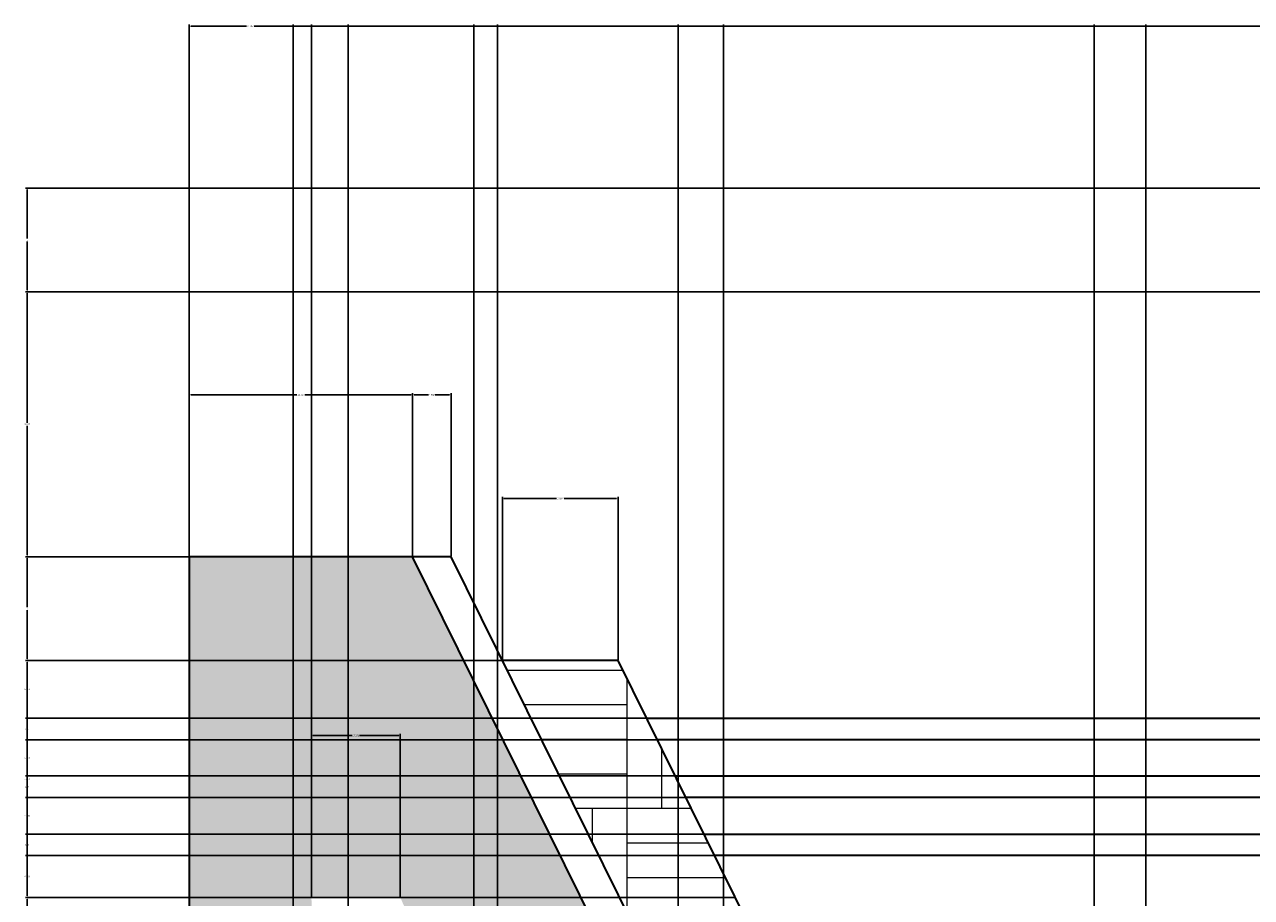
# Model space of a CAD drawing. Units: inches. Extents: x -9 to 389, y -55 to 344.
# Tile 3 of 5: x -9 to 133, y 243 to 344. Entities that reach past the tile are written whole.
import ezdxf

# ---------------------------------------------------------------- set-up
doc = ezdxf.new("R2010")
doc.units = ezdxf.units.IN
doc.header["$MEASUREMENT"] = 0
for name, color, linetype, lineweight in [('A-ANNO-DIMS', 2, 'Continuous', 18), ('A-ELEV', 7, 'Continuous', 35), ('A-ELEV-PATT', 8, 'Continuous', 13), ('A-ROOF', 1, 'Continuous', 35), ('A-ROOF-PATT', 8, 'Continuous', 13)]:
    doc.layers.add(name, color=color, linetype=linetype, lineweight=lineweight)
doc.styles.get("Standard").update_dxf_attribs({"font": 'arial.ttf'})
doc.dimstyles.get("Standard").update_dxf_attribs({"dimtxt": 0.18, "dimasz": 0.18, "dimexe": 0.18, "dimexo": 0.0625, "dimgap": 0.09, "dimtad": 0, "dimtih": 1, "dimtoh": 1, "dimdec": 4, "dimzin": 0, "dimdsep": 46, "dimtxsty": 'Standard', "dimcen": 0.09, "dimadec": 0, "dimazin": 0, "dimtfac": 1, "dimtdec": 4, "dimtofl": 0, "dimtmove": 0, "dimatfit": 3, "dimfxl": 1, "dimtolj": 1, "dimtzin": 0, "dimarcsym": 0})

# ---------------------------------------------------------------- blocks, each defined once
blk = doc.blocks.new('*D1')
at = {"layer": 'A-ANNO-DIMS', "color": 0, "lineweight": -2, "transparency": 16777216}
for p, q in [((9.65, 282.26), (9.65, 343.8)), ((9.83, 343.62), (16.26, 343.62)), ((23.59, 343.62), (17.17, 343.62)), ((23.77, 242.83), (23.77, 343.8))]:
    blk.add_line(p, q, dxfattribs=at)
at = {"layer": 'A-ANNO-DIMS', "color": 0, "transparency": 16777216}
for points in [[(9.83, 343.65), (9.83, 343.59), (9.65, 343.62)], [(23.59, 343.65), (23.59, 343.59), (23.77, 343.62)]]:
    blk.add_solid(points, dxfattribs=at)
at = {"layer": 'Defpoints', "color": 0, "transparency": 16777216}
for p in [(23.77, 343.62), (9.65, 282.2), (23.77, 242.77)]:
    blk.add_point(p, dxfattribs=at)
at = {"layer": 'A-ANNO-DIMS', "color": 0, "transparency": 16777216, "insert": (16.71, 343.62), "char_height": 0.18, "attachment_point": 5}
blk.add_mtext('\\A1;14.118', dxfattribs=at)
blk = doc.blocks.new('*D2')
at = {"layer": 'A-ANNO-DIMS', "color": 0, "lineweight": -2, "transparency": 16777216}
for p, q in [((23.77, 242.83), (23.77, 343.8)), ((23.95, 343.62), (25.5, 343.62)), ((27.83, 343.62), (26.29, 343.62)), ((28.01, 157.47), (28.01, 343.8))]:
    blk.add_line(p, q, dxfattribs=at)
at = {"layer": 'A-ANNO-DIMS', "color": 0, "transparency": 16777216}
for points in [[(23.95, 343.65), (23.95, 343.59), (23.77, 343.62)], [(27.83, 343.65), (27.83, 343.59), (28.01, 343.62)]]:
    blk.add_solid(points, dxfattribs=at)
at = {"layer": 'Defpoints', "color": 0, "transparency": 16777216}
for p in [(28.01, 343.62), (23.77, 242.77), (28.01, 157.4)]:
    blk.add_point(p, dxfattribs=at)
at = {"layer": 'A-ANNO-DIMS', "color": 0, "transparency": 16777216, "insert": (25.89, 343.62), "char_height": 0.18, "attachment_point": 5}
blk.add_mtext('\\A1;4.244', dxfattribs=at)
blk = doc.blocks.new('*D3')
at = {"layer": 'A-ANNO-DIMS', "color": 0, "lineweight": -2, "transparency": 16777216}
for p, q in [((28.01, 157.47), (28.01, 343.8)), ((28.19, 343.62), (49.26, 343.62)), ((71.27, 343.62), (50.2, 343.62)), ((71.45, 157.47), (71.45, 343.8))]:
    blk.add_line(p, q, dxfattribs=at)
at = {"layer": 'A-ANNO-DIMS', "color": 0, "transparency": 16777216}
for points in [[(28.19, 343.65), (28.19, 343.59), (28.01, 343.62)], [(71.27, 343.65), (71.27, 343.59), (71.45, 343.62)]]:
    blk.add_solid(points, dxfattribs=at)
at = {"layer": 'Defpoints', "color": 0, "transparency": 16777216}
for p in [(71.45, 343.62), (28.01, 157.4), (71.45, 157.4)]:
    blk.add_point(p, dxfattribs=at)
at = {"layer": 'A-ANNO-DIMS', "color": 0, "transparency": 16777216, "insert": (49.73, 343.62), "char_height": 0.18, "attachment_point": 5}
blk.add_mtext('\\A1;43.435', dxfattribs=at)
blk = doc.blocks.new('*D4')
at = {"layer": 'A-ANNO-DIMS', "color": 0, "lineweight": -2, "transparency": 16777216}
for p, q in [((71.45, 157.47), (71.45, 343.8)), ((71.63, 343.62), (119.03, 343.62)), ((167.08, 343.62), (119.68, 343.62)), ((167.26, 324.93), (167.26, 343.8))]:
    blk.add_line(p, q, dxfattribs=at)
at = {"layer": 'A-ANNO-DIMS', "color": 0, "transparency": 16777216}
for points in [[(71.63, 343.65), (71.63, 343.59), (71.45, 343.62)], [(167.08, 343.65), (167.08, 343.59), (167.26, 343.62)]]:
    blk.add_solid(points, dxfattribs=at)
at = {"layer": 'Defpoints', "color": 0, "transparency": 16777216}
for p in [(167.26, 343.62), (167.26, 324.87), (71.45, 157.4)]:
    blk.add_point(p, dxfattribs=at)
at = {"layer": 'A-ANNO-DIMS', "color": 0, "transparency": 16777216, "insert": (119.35, 343.62), "char_height": 0.18, "attachment_point": 5}
blk.add_mtext('\\A1;95.8', dxfattribs=at)
blk = doc.blocks.new('*D16')
at = {"layer": 'A-ANNO-DIMS', "color": 0, "lineweight": -2, "transparency": 16777216}
for p, q in [((21.65, 14.83), (21.65, 343.8)), ((21.83, 343.62), (31.64, 343.62)), ((42.37, 343.62), (32.57, 343.62)), ((42.55, 14.83), (42.55, 343.8))]:
    blk.add_line(p, q, dxfattribs=at)
at = {"layer": 'A-ANNO-DIMS', "color": 0, "transparency": 16777216}
for points in [[(21.83, 343.65), (21.83, 343.59), (21.65, 343.62)], [(42.37, 343.65), (42.37, 343.59), (42.55, 343.62)]]:
    blk.add_solid(points, dxfattribs=at)
at = {"layer": 'Defpoints', "color": 0, "transparency": 16777216}
for p in [(42.55, 343.62), (21.65, 14.77), (42.55, 14.77)]:
    blk.add_point(p, dxfattribs=at)
at = {"layer": 'A-ANNO-DIMS', "color": 0, "transparency": 16777216, "insert": (32.1, 343.62), "char_height": 0.18, "attachment_point": 5}
blk.add_mtext('\\A1;20.896', dxfattribs=at)
blk = doc.blocks.new('*D17')
at = {"layer": 'A-ANNO-DIMS', "color": 0, "lineweight": -2, "transparency": 16777216}
for p, q in [((42.55, 14.83), (42.55, 343.8)), ((42.73, 343.62), (43.61, 343.62)), ((45.14, 343.62), (44.26, 343.62)), ((45.32, 14.83), (45.32, 343.8))]:
    blk.add_line(p, q, dxfattribs=at)
at = {"layer": 'A-ANNO-DIMS', "color": 0, "transparency": 16777216}
for points in [[(42.73, 343.65), (42.73, 343.59), (42.55, 343.62)], [(45.14, 343.65), (45.14, 343.59), (45.32, 343.62)]]:
    blk.add_solid(points, dxfattribs=at)
at = {"layer": 'Defpoints', "color": 0, "transparency": 16777216}
for p in [(45.32, 343.62), (42.55, 14.77), (45.32, 14.77)]:
    blk.add_point(p, dxfattribs=at)
at = {"layer": 'A-ANNO-DIMS', "color": 0, "transparency": 16777216, "insert": (43.93, 343.62), "char_height": 0.18, "attachment_point": 5}
blk.add_mtext('\\A1;2.77', dxfattribs=at)
blk = doc.blocks.new('*D18')
at = {"layer": 'A-ANNO-DIMS', "color": 0, "lineweight": -2, "transparency": 16777216}
for p, q in [((45.32, 14.83), (45.32, 343.8)), ((45.5, 343.62), (55.3, 343.62)), ((66.03, 343.62), (56.23, 343.62)), ((66.21, 14.83), (66.21, 343.8))]:
    blk.add_line(p, q, dxfattribs=at)
at = {"layer": 'A-ANNO-DIMS', "color": 0, "transparency": 16777216}
for points in [[(45.5, 343.65), (45.5, 343.59), (45.32, 343.62)], [(66.03, 343.65), (66.03, 343.59), (66.21, 343.62)]]:
    blk.add_solid(points, dxfattribs=at)
at = {"layer": 'Defpoints', "color": 0, "transparency": 16777216}
for p in [(66.21, 343.62), (45.32, 14.77), (66.21, 14.77)]:
    blk.add_point(p, dxfattribs=at)
at = {"layer": 'A-ANNO-DIMS', "color": 0, "transparency": 16777216, "insert": (55.77, 343.62), "char_height": 0.18, "attachment_point": 5}
blk.add_mtext('\\A1;20.896', dxfattribs=at)
blk = doc.blocks.new('*D19')
at = {"layer": 'A-ANNO-DIMS', "color": 0, "lineweight": -2, "transparency": 16777216}
for p, q in [((66.21, 14.83), (66.21, 343.8)), ((66.39, 343.62), (109.71, 343.62)), ((153.81, 343.62), (110.5, 343.62)), ((153.99, 14.83), (153.99, 343.8))]:
    blk.add_line(p, q, dxfattribs=at)
at = {"layer": 'A-ANNO-DIMS', "color": 0, "transparency": 16777216}
for points in [[(66.39, 343.65), (66.39, 343.59), (66.21, 343.62)], [(153.81, 343.65), (153.81, 343.59), (153.99, 343.62)]]:
    blk.add_solid(points, dxfattribs=at)
at = {"layer": 'Defpoints', "color": 0, "transparency": 16777216}
for p in [(153.99, 343.62), (66.21, 14.77), (153.99, 14.77)]:
    blk.add_point(p, dxfattribs=at)
at = {"layer": 'A-ANNO-DIMS', "color": 0, "transparency": 16777216, "insert": (110.1, 343.62), "char_height": 0.18, "attachment_point": 5}
blk.add_mtext('\\A1;87.77', dxfattribs=at)
blk = doc.blocks.new('*D25')
at = {"layer": 'A-ANNO-DIMS', "color": 0, "lineweight": -2, "transparency": 16777216}
for p, q in [((23.71, 242.77), (-9.28, 242.77)), ((-9.1, 242.59), (-9.1, 200.27)), ((-9.1, 157.58), (-9.1, 199.9)), ((27.95, 157.4), (-9.28, 157.4))]:
    blk.add_line(p, q, dxfattribs=at)
at = {"layer": 'A-ANNO-DIMS', "color": 0, "transparency": 16777216}
for points in [[(-9.13, 242.59), (-9.07, 242.59), (-9.1, 242.77)], [(-9.13, 157.58), (-9.07, 157.58), (-9.1, 157.4)]]:
    blk.add_solid(points, dxfattribs=at)
at = {"layer": 'Defpoints', "color": 0, "transparency": 16777216}
for p in [(-9.1, 242.77), (23.77, 242.77), (28.01, 157.4)]:
    blk.add_point(p, dxfattribs=at)
at = {"layer": 'A-ANNO-DIMS', "color": 0, "transparency": 16777216, "insert": (-9.1, 200.09), "char_height": 0.18, "attachment_point": 5}
blk.add_mtext('\\A1;85.36', dxfattribs=at)
blk = doc.blocks.new('*D26')
at = {"layer": 'A-ANNO-DIMS', "color": 0, "lineweight": -2, "transparency": 16777216}
for p, q in [((59.2, 270.2), (-9.28, 270.2)), ((-9.1, 270.02), (-9.1, 256.67)), ((-9.1, 242.95), (-9.1, 256.3)), ((23.71, 242.77), (-9.28, 242.77))]:
    blk.add_line(p, q, dxfattribs=at)
at = {"layer": 'A-ANNO-DIMS', "color": 0, "transparency": 16777216}
for points in [[(-9.13, 270.02), (-9.07, 270.02), (-9.1, 270.2)], [(-9.13, 242.95), (-9.07, 242.95), (-9.1, 242.77)]]:
    blk.add_solid(points, dxfattribs=at)
at = {"layer": 'Defpoints', "color": 0, "transparency": 16777216}
for p in [(-9.1, 270.2), (59.26, 270.2), (23.77, 242.77)]:
    blk.add_point(p, dxfattribs=at)
at = {"layer": 'A-ANNO-DIMS', "color": 0, "transparency": 16777216, "insert": (-9.1, 256.48), "char_height": 0.18, "attachment_point": 5}
blk.add_mtext('\\A1;27.43', dxfattribs=at)
blk = doc.blocks.new('*D27')
at = {"layer": 'A-ANNO-DIMS', "color": 0, "lineweight": -2, "transparency": 16777216}
for p, q in [((9.59, 282.2), (-9.28, 282.2)), ((-9.1, 282.02), (-9.1, 276.38)), ((-9.1, 270.38), (-9.1, 276.02)), ((59.2, 270.2), (-9.28, 270.2))]:
    blk.add_line(p, q, dxfattribs=at)
at = {"layer": 'A-ANNO-DIMS', "color": 0, "transparency": 16777216}
for points in [[(-9.13, 282.02), (-9.07, 282.02), (-9.1, 282.2)], [(-9.13, 270.38), (-9.07, 270.38), (-9.1, 270.2)]]:
    blk.add_solid(points, dxfattribs=at)
at = {"layer": 'Defpoints', "color": 0, "transparency": 16777216}
for p in [(-9.1, 282.2), (9.65, 282.2), (59.26, 270.2)]:
    blk.add_point(p, dxfattribs=at)
at = {"layer": 'A-ANNO-DIMS', "color": 0, "transparency": 16777216, "insert": (-9.1, 276.2), "char_height": 0.18, "attachment_point": 5}
blk.add_mtext('\\A1;12', dxfattribs=at)
blk = doc.blocks.new('*D28')
at = {"layer": 'A-ANNO-DIMS', "color": 0, "lineweight": -2, "transparency": 16777216}
for p, q in [((160.42, 312.87), (-9.28, 312.87)), ((-9.1, 312.69), (-9.1, 297.72)), ((-9.1, 282.38), (-9.1, 297.35)), ((9.59, 282.2), (-9.28, 282.2))]:
    blk.add_line(p, q, dxfattribs=at)
at = {"layer": 'A-ANNO-DIMS', "color": 0, "transparency": 16777216}
for points in [[(-9.13, 312.69), (-9.07, 312.69), (-9.1, 312.87)], [(-9.13, 282.38), (-9.07, 282.38), (-9.1, 282.2)]]:
    blk.add_solid(points, dxfattribs=at)
at = {"layer": 'Defpoints', "color": 0, "transparency": 16777216}
for p in [(-9.1, 312.87), (160.49, 312.87), (9.65, 282.2)]:
    blk.add_point(p, dxfattribs=at)
at = {"layer": 'A-ANNO-DIMS', "color": 0, "transparency": 16777216, "insert": (-9.1, 297.54), "char_height": 0.18, "attachment_point": 5}
blk.add_mtext('\\A1;30.67', dxfattribs=at)
blk = doc.blocks.new('*D29')
at = {"layer": 'A-ANNO-DIMS', "color": 0, "lineweight": -2, "transparency": 16777216}
for p, q in [((369.59, 324.87), (-9.28, 324.87)), ((-9.1, 324.69), (-9.1, 319.05)), ((-9.1, 313.05), (-9.1, 318.69)), ((160.42, 312.87), (-9.28, 312.87))]:
    blk.add_line(p, q, dxfattribs=at)
at = {"layer": 'A-ANNO-DIMS', "color": 0, "transparency": 16777216}
for points in [[(-9.13, 324.69), (-9.07, 324.69), (-9.1, 324.87)], [(-9.13, 313.05), (-9.07, 313.05), (-9.1, 312.87)]]:
    blk.add_solid(points, dxfattribs=at)
at = {"layer": 'Defpoints', "color": 0, "transparency": 16777216}
for p in [(-9.1, 324.87), (369.65, 324.87), (160.49, 312.87)]:
    blk.add_point(p, dxfattribs=at)
at = {"layer": 'A-ANNO-DIMS', "color": 0, "transparency": 16777216, "insert": (-9.1, 318.87), "char_height": 0.18, "attachment_point": 5}
blk.add_mtext('\\A1;12', dxfattribs=at)
blk = doc.blocks.new('*D34')
at = {"layer": 'A-ANNO-DIMS', "color": 0, "lineweight": -2, "transparency": 16777216}
for p, q in [((9.65, 282.26), (9.65, 301.13)), ((9.83, 300.95), (22.1, 300.95)), ((35.3, 300.95), (23.03, 300.95)), ((35.48, 282.26), (35.48, 301.13))]:
    blk.add_line(p, q, dxfattribs=at)
at = {"layer": 'A-ANNO-DIMS', "color": 0, "transparency": 16777216}
for points in [[(9.83, 300.98), (9.83, 300.92), (9.65, 300.95)], [(35.3, 300.98), (35.3, 300.92), (35.48, 300.95)]]:
    blk.add_solid(points, dxfattribs=at)
at = {"layer": 'Defpoints', "color": 0, "transparency": 16777216}
for p in [(35.48, 300.95), (9.65, 282.2), (35.48, 282.2)]:
    blk.add_point(p, dxfattribs=at)
at = {"layer": 'A-ANNO-DIMS', "color": 0, "transparency": 16777216, "insert": (22.57, 300.95), "char_height": 0.18, "attachment_point": 5}
blk.add_mtext('\\A1;25.825', dxfattribs=at)
blk = doc.blocks.new('*D35')
at = {"layer": 'A-ANNO-DIMS', "color": 0, "lineweight": -2, "transparency": 16777216}
for p, q in [((35.48, 282.26), (35.48, 301.13)), ((35.66, 300.95), (37.31, 300.95)), ((39.76, 300.95), (38.11, 300.95)), ((39.94, 282.26), (39.94, 301.13))]:
    blk.add_line(p, q, dxfattribs=at)
at = {"layer": 'A-ANNO-DIMS', "color": 0, "transparency": 16777216}
for points in [[(35.66, 300.98), (35.66, 300.92), (35.48, 300.95)], [(39.76, 300.98), (39.76, 300.92), (39.94, 300.95)]]:
    blk.add_solid(points, dxfattribs=at)
at = {"layer": 'Defpoints', "color": 0, "transparency": 16777216}
for p in [(39.94, 300.95), (35.48, 282.2), (39.94, 282.2)]:
    blk.add_point(p, dxfattribs=at)
at = {"layer": 'A-ANNO-DIMS', "color": 0, "transparency": 16777216, "insert": (37.71, 300.95), "char_height": 0.18, "attachment_point": 5}
blk.add_mtext('\\A1;4.462', dxfattribs=at)
blk = doc.blocks.new('*D37')
at = {"layer": 'A-ANNO-DIMS', "color": 0, "lineweight": -2, "transparency": 16777216}
for p, q in [((45.87, 270.26), (45.87, 289.13)), ((46.05, 288.95), (52.11, 288.95)), ((59.08, 288.95), (53.02, 288.95)), ((59.26, 270.26), (59.26, 289.13))]:
    blk.add_line(p, q, dxfattribs=at)
at = {"layer": 'A-ANNO-DIMS', "color": 0, "transparency": 16777216}
for points in [[(46.05, 288.98), (46.05, 288.92), (45.87, 288.95)], [(59.08, 288.98), (59.08, 288.92), (59.26, 288.95)]]:
    blk.add_solid(points, dxfattribs=at)
at = {"layer": 'Defpoints', "color": 0, "transparency": 16777216}
for p in [(59.26, 288.95), (45.87, 270.2), (59.26, 270.2)]:
    blk.add_point(p, dxfattribs=at)
at = {"layer": 'A-ANNO-DIMS', "color": 0, "transparency": 16777216, "insert": (52.57, 288.95), "char_height": 0.18, "attachment_point": 5}
blk.add_mtext('\\A1;13.387', dxfattribs=at)
blk = doc.blocks.new('*D39')
at = {"layer": 'A-ANNO-DIMS', "color": 0, "lineweight": -2, "transparency": 16777216}
for p, q in [((23.77, 242.83), (23.77, 261.7)), ((23.95, 261.52), (28.48, 261.52)), ((33.88, 261.52), (29.35, 261.52)), ((34.06, 242.83), (34.06, 261.7))]:
    blk.add_line(p, q, dxfattribs=at)
at = {"layer": 'A-ANNO-DIMS', "color": 0, "transparency": 16777216}
for points in [[(23.95, 261.55), (23.95, 261.49), (23.77, 261.52)], [(33.88, 261.55), (33.88, 261.49), (34.06, 261.52)]]:
    blk.add_solid(points, dxfattribs=at)
at = {"layer": 'Defpoints', "color": 0, "transparency": 16777216}
for p in [(34.06, 261.52), (23.77, 242.77), (34.06, 242.77)]:
    blk.add_point(p, dxfattribs=at)
at = {"layer": 'A-ANNO-DIMS', "color": 0, "transparency": 16777216, "insert": (28.92, 261.52), "char_height": 0.18, "attachment_point": 5}
blk.add_mtext('\\A1;10.291', dxfattribs=at)
blk = doc.blocks.new('*D49')
at = {"layer": 'A-ANNO-DIMS', "color": 0, "lineweight": -2, "transparency": 16777216}
for p, q in [((72.76, 242.77), (-9.28, 242.77)), ((-9.1, 242.59), (-9.1, 232.95)), ((-9.1, 222.95), (-9.1, 232.59)), ((82.66, 222.77), (-9.28, 222.77))]:
    blk.add_line(p, q, dxfattribs=at)
at = {"layer": 'A-ANNO-DIMS', "color": 0, "transparency": 16777216}
for points in [[(-9.13, 242.59), (-9.07, 242.59), (-9.1, 242.77)], [(-9.13, 222.95), (-9.07, 222.95), (-9.1, 222.77)]]:
    blk.add_solid(points, dxfattribs=at)
at = {"layer": 'Defpoints', "color": 0, "transparency": 16777216}
for p in [(-9.1, 242.77), (72.83, 242.77), (82.72, 222.77)]:
    blk.add_point(p, dxfattribs=at)
at = {"layer": 'A-ANNO-DIMS', "color": 0, "transparency": 16777216, "insert": (-9.1, 232.77), "char_height": 0.18, "attachment_point": 5}
blk.add_mtext('\\A1;20', dxfattribs=at)
blk = doc.blocks.new('*D50')
at = {"layer": 'A-ANNO-DIMS', "color": 0, "lineweight": -2, "transparency": 16777216}
for p, q in [((70.37, 247.61), (-9.28, 247.61)), ((-9.1, 247.43), (-9.1, 245.37)), ((-9.1, 242.95), (-9.1, 245.01)), ((72.76, 242.77), (-9.28, 242.77))]:
    blk.add_line(p, q, dxfattribs=at)
at = {"layer": 'A-ANNO-DIMS', "color": 0, "transparency": 16777216}
for points in [[(-9.13, 247.43), (-9.07, 247.43), (-9.1, 247.61)], [(-9.13, 242.95), (-9.07, 242.95), (-9.1, 242.77)]]:
    blk.add_solid(points, dxfattribs=at)
at = {"layer": 'Defpoints', "color": 0, "transparency": 16777216}
for p in [(-9.1, 247.61), (70.43, 247.61), (72.83, 242.77)]:
    blk.add_point(p, dxfattribs=at)
at = {"layer": 'A-ANNO-DIMS', "color": 0, "transparency": 16777216, "insert": (-9.1, 245.19), "char_height": 0.18, "attachment_point": 5}
blk.add_mtext('\\A1;4.843', dxfattribs=at)
blk = doc.blocks.new('*D51')
at = {"layer": 'A-ANNO-DIMS', "color": 0, "lineweight": -2, "transparency": 16777216}
for p, q in [((69.13, 250.11), (-9.28, 250.11)), ((-9.1, 249.93), (-9.1, 249.04)), ((-9.1, 247.79), (-9.1, 248.68)), ((70.37, 247.61), (-9.28, 247.61))]:
    blk.add_line(p, q, dxfattribs=at)
at = {"layer": 'A-ANNO-DIMS', "color": 0, "transparency": 16777216}
for points in [[(-9.13, 249.93), (-9.07, 249.93), (-9.1, 250.11)], [(-9.13, 247.79), (-9.07, 247.79), (-9.1, 247.61)]]:
    blk.add_solid(points, dxfattribs=at)
at = {"layer": 'Defpoints', "color": 0, "transparency": 16777216}
for p in [(-9.1, 250.11), (69.19, 250.11), (70.43, 247.61)]:
    blk.add_point(p, dxfattribs=at)
at = {"layer": 'A-ANNO-DIMS', "color": 0, "transparency": 16777216, "insert": (-9.1, 248.86), "char_height": 0.18, "attachment_point": 5}
blk.add_mtext('\\A1;2.50', dxfattribs=at)
blk = doc.blocks.new('*D52')
at = {"layer": 'A-ANNO-DIMS', "color": 0, "lineweight": -2, "transparency": 16777216}
for p, q in [((67.05, 254.33), (-9.28, 254.33)), ((-9.1, 254.15), (-9.1, 252.4)), ((-9.1, 250.29), (-9.1, 252.04)), ((69.13, 250.11), (-9.28, 250.11))]:
    blk.add_line(p, q, dxfattribs=at)
at = {"layer": 'A-ANNO-DIMS', "color": 0, "transparency": 16777216}
for points in [[(-9.13, 254.15), (-9.07, 254.15), (-9.1, 254.33)], [(-9.13, 250.29), (-9.07, 250.29), (-9.1, 250.11)]]:
    blk.add_solid(points, dxfattribs=at)
at = {"layer": 'Defpoints', "color": 0, "transparency": 16777216}
for p in [(-9.1, 254.33), (67.11, 254.33), (69.19, 250.11)]:
    blk.add_point(p, dxfattribs=at)
at = {"layer": 'A-ANNO-DIMS', "color": 0, "transparency": 16777216, "insert": (-9.1, 252.22), "char_height": 0.18, "attachment_point": 5}
blk.add_mtext('\\A1;4.216', dxfattribs=at)
blk = doc.blocks.new('*D53')
at = {"layer": 'A-ANNO-DIMS', "color": 0, "lineweight": -2, "transparency": 16777216}
for p, q in [((65.81, 256.83), (-9.28, 256.83)), ((-9.1, 256.65), (-9.1, 255.76)), ((67.05, 254.33), (-9.28, 254.33)), ((-9.1, 254.51), (-9.1, 255.4))]:
    blk.add_line(p, q, dxfattribs=at)
at = {"layer": 'A-ANNO-DIMS', "color": 0, "transparency": 16777216}
for points in [[(-9.13, 256.65), (-9.07, 256.65), (-9.1, 256.83)], [(-9.13, 254.51), (-9.07, 254.51), (-9.1, 254.33)]]:
    blk.add_solid(points, dxfattribs=at)
at = {"layer": 'Defpoints', "color": 0, "transparency": 16777216}
for p in [(-9.1, 256.83), (65.87, 256.83), (67.11, 254.33)]:
    blk.add_point(p, dxfattribs=at)
at = {"layer": 'A-ANNO-DIMS', "color": 0, "transparency": 16777216, "insert": (-9.1, 255.58), "char_height": 0.18, "attachment_point": 5}
blk.add_mtext('\\A1;2.50', dxfattribs=at)
blk = doc.blocks.new('*D54')
at = {"layer": 'A-ANNO-DIMS', "color": 0, "lineweight": -2, "transparency": 16777216}
for p, q in [((63.74, 261.01), (-9.28, 261.01)), ((-9.1, 260.83), (-9.1, 259.11)), ((-9.1, 257.01), (-9.1, 258.74)), ((65.81, 256.83), (-9.28, 256.83))]:
    blk.add_line(p, q, dxfattribs=at)
at = {"layer": 'A-ANNO-DIMS', "color": 0, "transparency": 16777216}
for points in [[(-9.13, 260.83), (-9.07, 260.83), (-9.1, 261.01)], [(-9.13, 257.01), (-9.07, 257.01), (-9.1, 256.83)]]:
    blk.add_solid(points, dxfattribs=at)
at = {"layer": 'Defpoints', "color": 0, "transparency": 16777216}
for p in [(-9.1, 261.01), (63.8, 261.01), (65.87, 256.83)]:
    blk.add_point(p, dxfattribs=at)
at = {"layer": 'A-ANNO-DIMS', "color": 0, "transparency": 16777216, "insert": (-9.1, 258.92), "char_height": 0.18, "attachment_point": 5}
blk.add_mtext('\\A1;4.183', dxfattribs=at)
blk = doc.blocks.new('*D55')
at = {"layer": 'A-ANNO-DIMS', "color": 0, "lineweight": -2, "transparency": 16777216}
for p, q in [((62.5, 263.52), (-9.28, 263.52)), ((-9.1, 263.34), (-9.1, 262.45)), ((-9.1, 261.19), (-9.1, 262.08)), ((63.74, 261.01), (-9.28, 261.01))]:
    blk.add_line(p, q, dxfattribs=at)
at = {"layer": 'A-ANNO-DIMS', "color": 0, "transparency": 16777216}
for points in [[(-9.13, 263.34), (-9.07, 263.34), (-9.1, 263.52)], [(-9.13, 261.19), (-9.07, 261.19), (-9.1, 261.01)]]:
    blk.add_solid(points, dxfattribs=at)
at = {"layer": 'Defpoints', "color": 0, "transparency": 16777216}
for p in [(-9.1, 263.52), (62.57, 263.52), (63.8, 261.01)]:
    blk.add_point(p, dxfattribs=at)
at = {"layer": 'A-ANNO-DIMS', "color": 0, "transparency": 16777216, "insert": (-9.1, 262.27), "char_height": 0.18, "attachment_point": 5}
blk.add_mtext('\\A1;2.50', dxfattribs=at)
blk = doc.blocks.new('*D56')
at = {"layer": 'A-ANNO-DIMS', "color": 0, "lineweight": -2, "transparency": 16777216}
for p, q in [((59.2, 270.2), (-9.28, 270.2)), ((-9.1, 270.02), (-9.1, 267.04)), ((-9.1, 263.7), (-9.1, 266.68)), ((62.5, 263.52), (-9.28, 263.52))]:
    blk.add_line(p, q, dxfattribs=at)
at = {"layer": 'A-ANNO-DIMS', "color": 0, "transparency": 16777216}
for points in [[(-9.13, 270.02), (-9.07, 270.02), (-9.1, 270.2)], [(-9.13, 263.7), (-9.07, 263.7), (-9.1, 263.52)]]:
    blk.add_solid(points, dxfattribs=at)
at = {"layer": 'Defpoints', "color": 0, "transparency": 16777216}
for p in [(-9.1, 270.2), (59.26, 270.2), (62.57, 263.52)]:
    blk.add_point(p, dxfattribs=at)
at = {"layer": 'A-ANNO-DIMS', "color": 0, "transparency": 16777216, "insert": (-9.1, 266.86), "char_height": 0.18, "attachment_point": 5}
blk.add_mtext('\\A1;6.683', dxfattribs=at)
blk = doc.blocks.new('*D57')
at = {"layer": 'A-ANNO-DIMS', "color": 0, "lineweight": -2, "transparency": 16777216}
for p, q in [((114.32, 122.83), (114.32, 343.8)), ((114.5, 343.62), (116.93, 343.62)), ((120.12, 343.62), (117.69, 343.62)), ((120.3, 146.83), (120.3, 343.8))]:
    blk.add_line(p, q, dxfattribs=at)
at = {"layer": 'A-ANNO-DIMS', "color": 0, "transparency": 16777216}
for points in [[(114.5, 343.65), (114.5, 343.59), (114.32, 343.62)], [(120.12, 343.65), (120.12, 343.59), (120.3, 343.62)]]:
    blk.add_solid(points, dxfattribs=at)
at = {"layer": 'Defpoints', "color": 0, "transparency": 16777216}
for p in [(120.3, 343.62), (120.3, 146.77), (114.32, 122.77)]:
    blk.add_point(p, dxfattribs=at)
at = {"layer": 'A-ANNO-DIMS', "color": 0, "transparency": 16777216, "insert": (117.31, 343.62), "char_height": 0.18, "attachment_point": 5}
blk.add_mtext('\\A1;5.981', dxfattribs=at)
blk = doc.blocks.new('*D58')
at = {"layer": 'A-ANNO-DIMS', "color": 0, "lineweight": -2, "transparency": 16777216}
for p, q in [((120.3, 146.83), (120.3, 343.8)), ((120.48, 343.62), (131.33, 343.62)), ((143.12, 343.62), (132.26, 343.62)), ((143.3, 146.83), (143.3, 343.8))]:
    blk.add_line(p, q, dxfattribs=at)
at = {"layer": 'A-ANNO-DIMS', "color": 0, "transparency": 16777216}
for points in [[(120.48, 343.65), (120.48, 343.59), (120.3, 343.62)], [(143.12, 343.65), (143.12, 343.59), (143.3, 343.62)]]:
    blk.add_solid(points, dxfattribs=at)
at = {"layer": 'Defpoints', "color": 0, "transparency": 16777216}
for p in [(143.3, 343.62), (120.3, 146.77), (143.3, 146.77)]:
    blk.add_point(p, dxfattribs=at)
at = {"layer": 'A-ANNO-DIMS', "color": 0, "transparency": 16777216, "insert": (131.8, 343.62), "char_height": 0.18, "attachment_point": 5}
blk.add_mtext('\\A1;22.994', dxfattribs=at)

msp = doc.modelspace()

# ---------------------------------------------------------------- hatches: boundary and pattern name
at = {"layer": 'A-ELEV-PATT'}
h = msp.add_hatch(color=256, dxfattribs=at)
h.dxf.hatch_style = 1
h.paths.add_polyline_path([(35.4778, 282.2003), (9.6533, 282.2003), (9.6533, 122.7681), (114.32, 122.7681)])
h.paths.add_polyline_path([(28.0148, 157.4044), (23.771, 242.7681), (34.0623, 242.7681), (71.4494, 157.4044)], flags=16)
at = {"layer": 'A-ROOF-PATT'}
h = msp.add_hatch(dxfattribs=at)
h.set_pattern_fill('AR-PARQ1', color=256, scale=2)
h.set_pattern_definition([(90, (-83.73, -34.93), (-24, 24), [24, -24]), (90, (-79.73, -34.93), (-24, 24), [24, -24]), (90, (-75.73, -34.93), (-24, 24), [24, -24]), (90, (-71.73, -34.93), (-24, 24), [24, -24]), (90, (-67.73, -34.93), (-24, 24), [24, -24]), (90, (-63.73, -34.93), (-24, 24), [24, -24]), (90, (-59.73, -34.93), (-24, 24), [24, -24]), (0, (-83.73, -10.93), (24, -24), [24, -24]), (0, (-83.73, -6.93), (24, -24), [24, -24]), (0, (-83.73, -2.93), (24, -24), [24, -24]), (0, (-83.73, 1.07), (24, -24), [24, -24]), (0, (-83.73, 5.07), (24, -24), [24, -24]), (0, (-83.73, 9.07), (24, -24), [24, -24]), (0, (-83.73, 13.07), (24, -24), [24, -24])])
h.paths.add_polyline_path([(59.2615, 270.2003), (45.8744, 270.2003), (116.6802, 127.0192), (130.2035, 126.7437)])
h.paths.add_polyline_path([(174.5076, 312.8713), (160.4864, 312.8713), (271.5791, 129.0492), (285.7644, 128.7778)])

# ---------------------------------------------------------------- linework, layer by layer
at = {"layer": 'A-ELEV'}
for p, q in [((39.9402, 282.2003), (9.6533, 282.2003)), ((9.6533, 282.2003), (9.6533, 122.7681))]:
    msp.add_line(p, q, dxfattribs=at)
for points in [[(62.5664, 263.5172), (190.3135, 263.5172)], [(191.8259, 261.0148), (191.8259, 261.0148), (63.8039, 261.0148)], [(65.8726, 256.8316), (194.354, 256.8316)], [(195.8663, 254.3292), (195.8663, 254.3292), (67.1101, 254.3292)], [(69.1949, 250.1134), (198.4141, 250.1134)], [(199.9265, 247.611), (199.9265, 247.611), (70.4324, 247.611)]]:
    msp.add_lwpolyline(points, dxfattribs=at)
at = {"layer": 'A-ROOF'}
for p, q in [((114.32, 122.7681), (35.4778, 282.2003)), ((118.7824, 122.7681), (39.9402, 282.2003)), ((59.2615, 270.2003), (45.8744, 270.2003)), ((130.2035, 126.7437), (59.2615, 270.2003))]:
    msp.add_line(p, q, dxfattribs=at)

# ---------------------------------------------------------------- dimensions: what is measured, and where the dimension line sits
at = {"layer": 'A-ANNO-DIMS'}
for base, p1, p2, override, picture, middle in [((23.771, 343.6213), (9.6533, 282.2003), (23.771, 242.7681), {"dimdec": 3, "dimlfac": 1, "dimrnd": 0, "dimzin": 0, "dimdsep": 46, "dimlunit": 2}, '*D1', (16.7122, 343.6213)), ((42.5492, 343.6213), (21.6533, 14.7681), (42.5492, 14.7681), {"dimdec": 3, "dimlfac": 1, "dimrnd": 0, "dimzin": 0, "dimdsep": 46, "dimlunit": 2}, '*D16', (32.1012, 343.6213)), ((28.0148, 343.6213), (23.771, 242.7681), (28.0148, 157.4044), {"dimdec": 3, "dimlfac": 1, "dimrnd": 0, "dimzin": 0, "dimdsep": 46, "dimlunit": 2}, '*D2', (25.8929, 343.6213)), ((71.4494, 343.6213), (28.0148, 157.4044), (71.4494, 157.4044), {"dimdec": 3, "dimlfac": 1, "dimrnd": 0, "dimzin": 0, "dimdsep": 46, "dimlunit": 2}, '*D3', (49.7321, 343.6213)), ((45.3188, 343.6213), (42.5492, 14.7681), (45.3188, 14.7681), {"dimdec": 2, "dimlfac": 1, "dimrnd": 0, "dimzin": 0, "dimdsep": 46, "dimlunit": 2}, '*D17', (43.934, 343.6213)), ((66.2148, 343.6213), (45.3188, 14.7681), (66.2148, 14.7681), {"dimdec": 3, "dimlfac": 1, "dimrnd": 0, "dimzin": 0, "dimdsep": 46, "dimlunit": 2}, '*D18', (55.7668, 343.6213)), ((153.9877, 343.6213), (66.2148, 14.7681), (153.9877, 14.7681), {"dimdec": 2, "dimlfac": 1, "dimrnd": 0, "dimzin": 0, "dimdsep": 46, "dimlunit": 2}, '*D19', (110.1012, 343.6213)), ((167.2555, 343.6213), (71.4494, 157.4044), (167.2555, 324.8713), {"dimdec": 1, "dimlfac": 1, "dimrnd": 0, "dimzin": 0, "dimdsep": 46, "dimlunit": 2}, '*D4', (119.3525, 343.6213)), ((120.3011, 343.6213), (114.32, 122.7681), (120.3011, 146.7681), {"dimdec": 3, "dimlfac": 1, "dimrnd": 0, "dimzin": 0, "dimdsep": 46, "dimlunit": 2}, '*D57', (117.3105, 343.6213)), ((143.2954, 343.6213), (120.3011, 146.7681), (143.2954, 146.7681), {"dimdec": 3, "dimlfac": 1, "dimrnd": 0, "dimzin": 0, "dimdsep": 46, "dimlunit": 2}, '*D58', (131.7983, 343.6213)), ((35.47778, 300.95029), (9.65327, 282.20029), (35.47778, 282.20029), {"dimdec": 3, "dimlfac": 1, "dimrnd": 0, "dimzin": 0, "dimdsep": 46, "dimlunit": 2}, '*D34', (22.56553, 300.95029)), ((39.9402, 300.9503), (35.4778, 282.2003), (39.9402, 282.2003), {"dimdec": 3, "dimlfac": 1, "dimrnd": 0, "dimzin": 0, "dimdsep": 46, "dimlunit": 2}, '*D35', (37.709, 300.9503)), ((34.0623, 261.5181), (23.771, 242.7681), (34.0623, 242.7681), {"dimdec": 3, "dimlfac": 1, "dimrnd": 0, "dimzin": 0, "dimdsep": 46, "dimlunit": 2}, '*D39', (28.9167, 261.5181))]:
    dim = msp.add_linear_dim(base=base, p1=p1, p2=p2, dimstyle='Standard', override=override, dxfattribs=at)
    dim.commit()
    dim.dimension.update_dxf_attribs({"geometry": picture, "text_midpoint": middle})
for base, p1, p2, angle, override, picture, middle in [((-9.0967, 324.8713), (160.4864, 312.8713), (369.6533, 324.8713), 90, {"dimdec": 0, "dimlfac": 1, "dimrnd": 0, "dimzin": 0, "dimdsep": 46, "dimlunit": 2}, '*D29', (-9.0967, 318.8713)), ((-9.0967, 312.8713), (9.6533, 282.2003), (160.4864, 312.8713), 90, {"dimdec": 2, "dimlfac": 1, "dimrnd": 0, "dimzin": 0, "dimdsep": 46, "dimlunit": 2}, '*D28', (-9.0967, 297.5358)), ((59.2615, 288.9503), (45.8744, 270.2003), (59.2615, 270.2003), 0, {"dimdec": 3, "dimlfac": 1, "dimrnd": 0, "dimzin": 0, "dimdsep": 46, "dimlunit": 2}, '*D37', (52.5679, 288.9503)), ((-9.0967, 282.2003), (59.2615, 270.2003), (9.6533, 282.2003), 90, {"dimdec": 0, "dimlfac": 1, "dimrnd": 0, "dimzin": 0, "dimdsep": 46, "dimlunit": 2}, '*D27', (-9.0967, 276.2003)), ((-9.0967, 270.2003), (23.771, 242.7681), (59.2615, 270.2003), 90, {"dimdec": 2, "dimlfac": 1, "dimrnd": 0, "dimzin": 0, "dimdsep": 46, "dimlunit": 2}, '*D26', (-9.0967, 256.4842)), ((-9.0967, 270.2003), (62.5664, 263.5172), (59.2615, 270.2003), 90, {"dimdec": 3, "dimlfac": 1, "dimrnd": 0, "dimzin": 0, "dimdsep": 46, "dimlunit": 2}, '*D56', (-9.0967, 266.8588)), ((-9.0967, 263.5172), (63.8039, 261.0148), (62.5664, 263.5172), 90, {"dimdec": 2, "dimlfac": 1, "dimrnd": 0, "dimzin": 0, "dimdsep": 46, "dimlunit": 2}, '*D55', (-9.0967, 262.266)), ((-9.0967, 261.0148), (65.8726, 256.8316), (63.8039, 261.0148), 90, {"dimdec": 3, "dimlfac": 1, "dimrnd": 0, "dimzin": 0, "dimdsep": 46, "dimlunit": 2}, '*D54', (-9.0967, 258.9232)), ((-9.0967, 256.8316), (67.1101, 254.3292), (65.8726, 256.8316), 90, {"dimdec": 2, "dimlfac": 1, "dimrnd": 0, "dimzin": 0, "dimdsep": 46, "dimlunit": 2}, '*D53', (-9.0967, 255.5804)), ((-9.0967, 254.3292), (69.1949, 250.1134), (67.1101, 254.3292), 90, {"dimdec": 3, "dimlfac": 1, "dimrnd": 0, "dimzin": 0, "dimdsep": 46, "dimlunit": 2}, '*D52', (-9.0967, 252.2213)), ((-9.0967, 250.1134), (70.4324, 247.611), (69.1949, 250.1134), 90, {"dimdec": 2, "dimlfac": 1, "dimrnd": 0, "dimzin": 0, "dimdsep": 46, "dimlunit": 2}, '*D51', (-9.0967, 248.8622)), ((-9.0967, 247.611), (72.8272, 242.7681), (70.4324, 247.611), 90, {"dimdec": 3, "dimlfac": 1, "dimrnd": 0, "dimzin": 0, "dimdsep": 46, "dimlunit": 2}, '*D50', (-9.0967, 245.1895)), ((-9.0967, 242.7681), (28.0148, 157.4044), (23.771, 242.7681), 90, {"dimdec": 2, "dimlfac": 1, "dimrnd": 0, "dimzin": 0, "dimdsep": 46, "dimlunit": 2}, '*D25', (-9.0967, 200.0863)), ((-9.0967, 242.7681), (82.7176, 222.7681), (72.8272, 242.7681), 90, {"dimdec": 0, "dimlfac": 1, "dimrnd": 0, "dimzin": 0, "dimdsep": 46, "dimlunit": 2}, '*D49', (-9.0967, 232.7681))]:
    dim = msp.add_linear_dim(base=base, p1=p1, p2=p2, angle=angle, dimstyle='Standard', override=override, dxfattribs=at)
    dim.commit()
    dim.dimension.update_dxf_attribs({"geometry": picture, "text_midpoint": middle})

doc.saveas('drawing.dxf')
